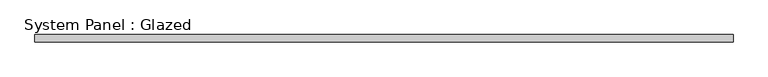
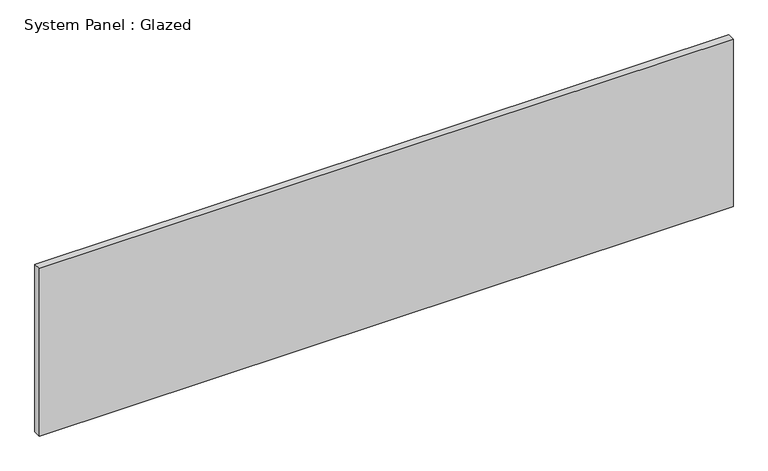
"""IFC4 building model written with IfcOpenShell, lengths in millimetres: plate geometry, System Panel : Glazed."""

from ifc_helpers import new_model, si_unit, origin, origin_with_axes, place, context, project, spatial, polyline, outline, extrude, source, transform, mapped, element, save


def system_panel_glazed_6011e45a(model_context):
    return source(origin(), model_context, "Body", "SweptSolid", [
        extrude(outline(polyline([(1171.575, 19.05), (-1171.575, 19.05), (-1171.575, 44.45), (1171.575, 44.45), (1171.575, 19.05)])), origin_with_axes(), (0.0, 0.0, 1.0), 598.1521067),
    ])


if __name__ == "__main__":
    model = new_model("IFC4")
    model_context = context("Model", 3, world=origin())
    ifc_project = project(units=[si_unit("LENGTHUNIT", "METRE", prefix="MILLI")], contexts=[model_context])
    site = spatial("IfcSite", under=ifc_project)
    building = spatial("IfcBuilding", under=site)
    placement = place(None, origin())
    system_panel_glazed_shape = system_panel_glazed_6011e45a(model_context)
    element("IfcPlate", 1, ObjectType="System Panel : Glazed", at=placement, inside=building, context=model_context, shape_type="MappedRepresentation", body=[
        mapped(system_panel_glazed_shape, transform((0.0, 0.0, 0.0), x_axis=(1.0, 0.0, 0.0), y_axis=(0.0, 1.0, 0.0), z_axis=(0.0, 0.0, 1.0))),
    ])
    save(model, "model.ifc")

# Revit data of these elements
# Type "System Panel : Glazed"
#   Construction Type Id = "GSP4R"
#   Analytic Construction = "1/8 in Pilkington single glazing"
#   Visual Light Transmittance = 0.9
#   Solar Heat Gain Coefficient = 0.86
#   Heat Transfer Coefficient (U) = 1.18115 BTU/(h·ft²·°F)
#   Define Thermal Properties by = 1
# Element 1 (IfcPlate, "System Panel : Glazed")
#   Materials on its faces: "Glass"
# Materials
#   "Glass": class "Glass", colour RGB 0 128 192, transparency 0.75, Description = "Soda Lime Glass", Cost = 0
